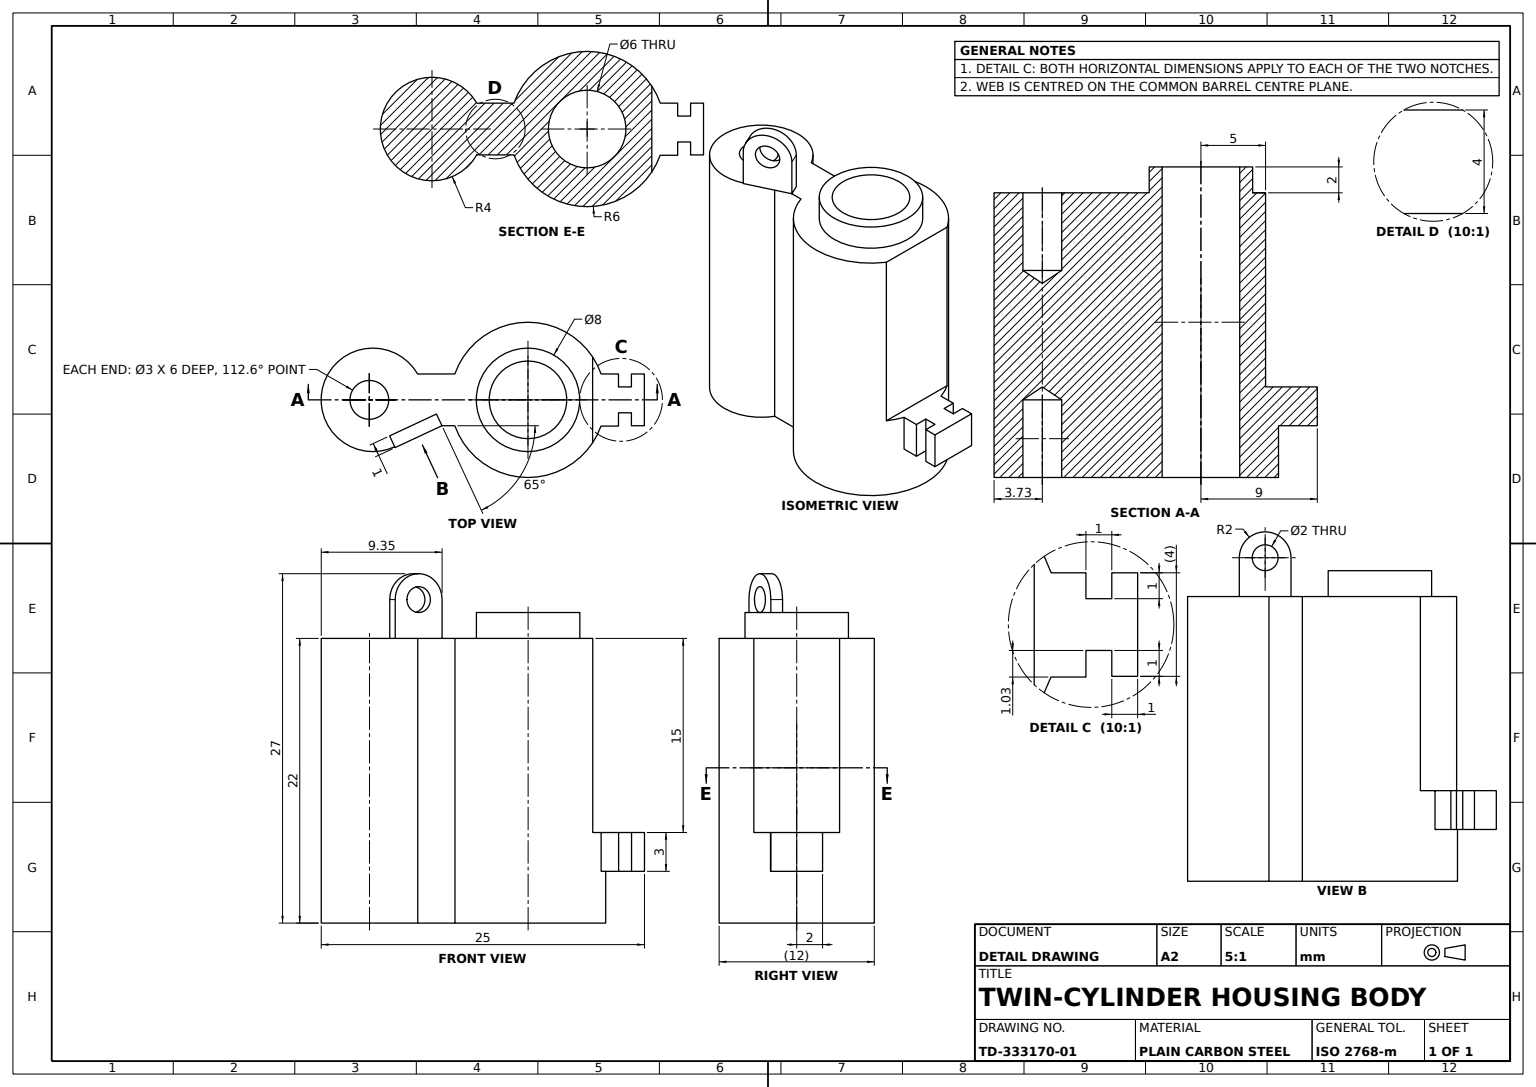
SolidWorks part; units mm, degrees
material "Plain Carbon Steel"
ref_plane "Front Plane" through (0, 0, 0) normal (0, 0, 1) x (1, 0, 0)
ref_plane "Top Plane" through (0, 0, 0) normal (0, 1, 0) x (1, 0, 0)
ref_plane "Right Plane" through (0, 0, 0) normal (1, 0, 0) x (0, 0, -1)
sketch "Twin Barrel Profile Sketch" plane through (0, 0, 0) normal (0, 1, 0) x (1, 0, 0)
  line L0 (0, 0) -> (9.0317, 0) construction
  line L1 (-8.5359, 2) -> (-5.6569, 2)
  line L3 (-8.5359, -2) -> (-5.6569, -2)
  line L5 (9.0317, 0) -> (9.0317, 8.711) construction
  arc A0 (-5.6569, -2) -> (-5.6569, 2) centre (0, 0) ccw
  arc A1 (-8.5359, 2) -> (-8.5359, -2) centre (-12, 0) ccw
  point P9 (-7.0964, 2)
  dimension "D1" = 12
  dimension "D2" = 8
  dimension "D3" = 12
  dimension "D4" = 4
  dimension "D5" = 9.0317
extrude "Twin Barrel Body" add sketch "Twin Barrel Profile Sketch" along normal blind 22
sketch "Eye Tab Sketch" plane through (0, 22, 0) normal (0, 1, 0) x (1, 0, 0)
  line L0 (-12, 0) -> (-8.3192, -7.8935) construction
  line L1 (-12, 0) -> (6.8611, 0) construction
  line L2 (-10.1874, 0.8452) -> (-6.5066, -7.0482) construction
  line L3 (-10.7017, -2.7842) -> (-8.8891, -1.9389)
  line L4 (-8.8891, -1.9389) -> (-7.0765, -1.0937)
  line L5 (-7.0765, -1.0937) -> (-6.6539, -2)
  line L6 (-6.6539, -2) -> (-10.2791, -3.6905)
  line L7 (-10.2791, -3.6905) -> (-10.7017, -2.7842)
  line L9 (-8.5359, -2) -> (-5.6569, -2) construction
  dimension "D1" = 65
  dimension "D3" = 1
  dimension "D4" = 4
  dimension "D2" = 2
extrude "Eye Tab" add sketch "Eye Tab Sketch" along normal blind 3
sketch "Eye Tab Boss Sketch" plane through (-0.4224, 0, -0.9058) normal (0.4226, 0, 0.9063) x (0.9063, 0, -0.4226)
  line L0 (-10.8757, 25) -> (-6.8757, 25) construction
  line L1 (-10.8757, 25) -> (-6.8757, 25)
  arc A0 (-6.8757, 25) -> (-10.8757, 25) centre (-8.8757, 25) ccw
extrude "Eye Tab Boss" add sketch "Eye Tab Boss Sketch" against normal blind 1
sketch "Eye Hole Sketch" plane through (-0.4224, 0, -0.9058) normal (0.4226, 0, 0.9063) x (0.9063, 0, -0.4226)
  circle A0 centre (-8.8757, 25) radius 1
  dimension "D1" = 2
extrude "Eye Hole Ø2" cut sketch "Eye Hole Sketch" against normal blind 1
sketch "Barrel Bore Profile Sketch" plane through (0, 0, 0) normal (0, 0, 1) x (1, 0, 0)
  line L0 (-12.2679, 22) -> (-12.2679, 15)
  line L1 (-8.5359, 22) -> (-16, 22) construction
  line L2 (-12.2679, 15) -> (-13.7679, 16)
  line L3 (-12.2679, 22) -> (-13.7679, 22)
  line L4 (-13.7679, 22) -> (-13.7679, 16)
  dimension "D1" = 7
  dimension "D4" = 1.5
  dimension "D5" = 6
revolve "Barrel Bore Cut" cut sketch "Barrel Bore Profile Sketch" angle 360 about L0
ref_plane "Barrel Mirror Plane" through (0, 11, 0) normal (0, 1, 0) x (1, 0, 0)
mirror "Barrel Bore Mirror" about plane through (0, 11, 0) normal (0, 1, 0) of "Barrel Bore Cut"
sketch "Collar Ring Sketch" plane through (0, 22, 0) normal (0, 1, 0) x (1, 0, 0)
  circle A0 centre (0, 0) radius 4
  circle A1 centre (0, 0) radius 3
  dimension "D1" = 8
  dimension "D2" = 6
extrude "Collar Ring Ø8" add sketch "Collar Ring Sketch" along normal blind 2
sketch "Collar Bore Sketch" plane through (0, 22, 0) normal (0, 1, 0) x (1, 0, 0)
  circle A0 centre (0, 0) radius 3 construction
  circle A1 centre (0, 0) radius 3
extrude "Collar Bore Cut" cut sketch "Collar Bore Sketch" against normal through all
ref_plane "Lug Offset Plane" through (0, 7, 0) normal (0, 1, 0) x (1, 0, 0)
sketch "Notched Lug Sketch" plane through (0, 7, 0) normal (0, 1, 0) x (1, 0, 0)
  line L0 (5, 3.3166) -> (5, -3.3166)
  line L1 (9, 2) -> (9, -2)
  line L2 (9, 2) -> (8, 2)
  line L3 (8, 2) -> (8, 1)
  line L4 (8, 1) -> (7, 1)
  line L5 (7, 1) -> (7, 2)
  line L6 (7, 2) -> (5.6569, 2)
  line L7 (9, -2) -> (8, -2)
  line L8 (8, -2) -> (8, -1)
  line L9 (8, -1) -> (7, -1)
  line L10 (7, -1) -> (7, -2.0277)
  line L11 (7, -2.0277) -> (5.647, -2.0277)
  arc A0 (-5.6569, -2) -> (-5.6569, 2) centre (0, 0) ccw construction
  arc A1 (5, -3.3166) -> (5.647, -2.0277) centre (0, 0) ccw
  arc A2 (5.6569, 2) -> (5, 3.3166) centre (0, 0) ccw
  dimension "D1" = 5
  dimension "D2" = 4
  dimension "D3" = 9
  dimension "D4" = 2
  dimension "D5" = 1
  dimension "D6" = 1
  dimension "D7" = 1
  dimension "D8" = 1
  dimension "D9" = 1
  dimension "D10" = 1
  dimension "D11" = 1.0277
extrude "Notched Lug" add sketch "Notched Lug Sketch" against normal blind 3
sketch "Lug Slot Sketch" plane through (0, 7, 0) normal (0, 1, 0) x (1, 0, 0)
  line L12 (5, 3.3166) -> (5, -3.3166)
  line L13 (5.647, -2.0277) -> (7, -2.0277)
  line L14 (7, -2.0277) -> (7, -1)
  line L15 (7, -1) -> (8, -1)
  line L16 (8, -1) -> (8, -2)
  line L17 (8, -2) -> (9, -2)
  line L18 (9, -2) -> (9, 2)
  line L19 (9, 2) -> (8, 2)
  line L20 (8, 2) -> (8, 1)
  line L21 (8, 1) -> (7, 1)
  line L22 (7, 1) -> (7, 2)
  line L23 (7, 2) -> (5.6569, 2)
  line L24 (5, 3.3166) -> (5, -3.3166)
  arc A2 (5, -3.3166) -> (5.647, -2.0277) centre (0, 0) ccw
  arc A3 (5.6569, 2) -> (5, 3.3166) centre (0, 0) ccw
  arc A4 (5, -3.3166) -> (5.647, -2.0277) centre (0, 0) ccw
  arc A5 (5.647, -2.0277) -> (5, 3.3166) centre (0, 0) ccw
  dimension "D1" = 0
extrude "Lug Slot Cut" cut sketch "Lug Slot Sketch" along normal through all
